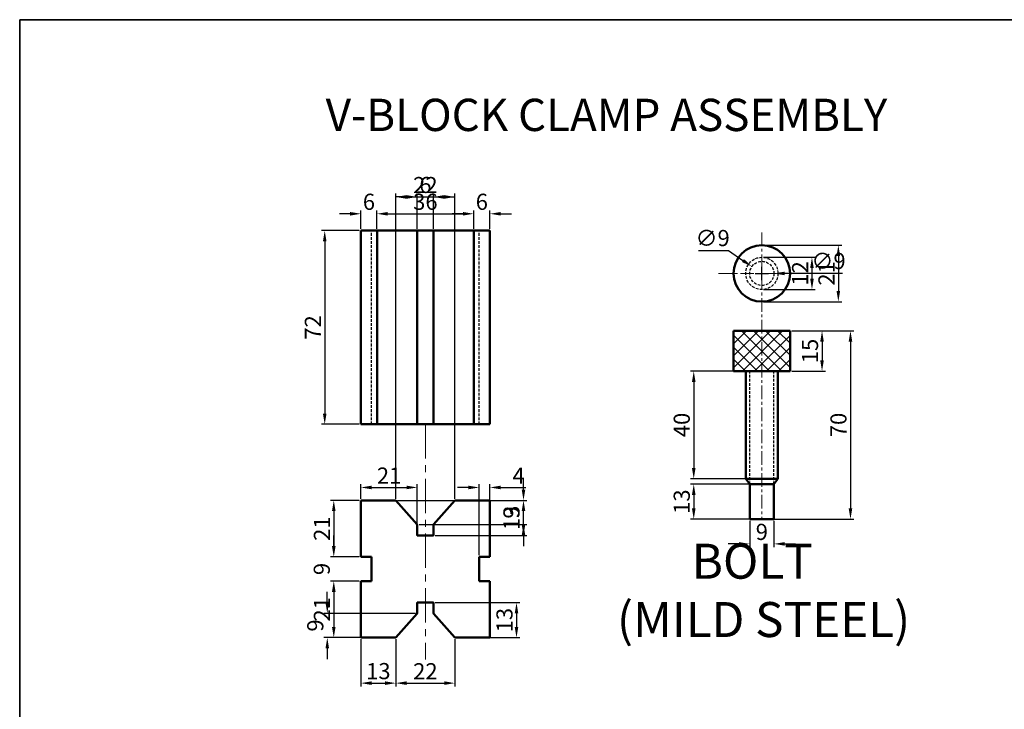
# Model space of a CAD drawing. Units: millimetres. Extents: x 0 to 624, y -214 to 340.
# Tile 2 of 3: x 0 to 366, y 84 to 340. Entities that reach past the tile are written whole.
import ezdxf

# ---------------------------------------------------------------- set-up
doc = ezdxf.new("R2010")
doc.units = ezdxf.units.MM
doc.header["$LTSCALE"] = 0.4
doc.linetypes.add('CENTER', pattern=[50.8, 31.75, -6.35, 6.35, -6.35])
doc.linetypes.add('HIDDEN', pattern=[9.525, 6.35, -3.175])
for name, color, linetype, lineweight in [('M-CNTR', 1, 'CENTER', 18), ('M-DIMS', 2, 'Continuous', 25), ('M-HATC', 8, 'Continuous', 18), ('M-HIDN', 4, 'HIDDEN', 25), ('M-OUTL', 7, 'Continuous', 50), ('M-TEXT', 3, 'Continuous', 25), ('M-TTLB', 7, 'Continuous', 35)]:
    doc.layers.add(name, color=color, linetype=linetype, lineweight=lineweight)
doc.styles.get("Standard").update_dxf_attribs({"font": 'arial.ttf'})
doc.dimstyles.new('ISO-25', dxfattribs={"dimtxt": 6, "dimasz": 4, "dimexe": 1.25, "dimexo": 0.625, "dimtad": 1, "dimtoh": 1, "dimtxsty": 'Standard', "dimcen": 2.5, "dimadec": 0, "dimazin": 0, "dimtfac": 1, "dimtofl": 0, "dimtmove": 0, "dimatfit": 3, "dimfxl": 1, "dimarcsym": 0})

# ---------------------------------------------------------------- blocks, each defined once
blk = doc.blocks.new('*D1')
at = {"layer": 'Defpoints', "color": 0, "transparency": 16777216}
for p in [(126.92, 110.45), (139.92, 110.45), (139.92, 93.53)]:
    blk.add_point(p, dxfattribs=at)
at = {"layer": 'M-DIMS', "color": 0, "lineweight": -2, "transparency": 16777216}
for p, q in [((126.92, 109.83), (126.92, 92.28)), ((139.92, 109.83), (139.92, 92.28)), ((130.92, 93.53), (135.92, 93.53))]:
    blk.add_line(p, q, dxfattribs=at)
at = {"layer": 'M-DIMS', "color": 0, "transparency": 16777216}
for points in [[(130.92, 94.2), (130.92, 92.86), (126.92, 93.53)], [(135.92, 94.2), (135.92, 92.86), (139.92, 93.53)]]:
    blk.add_solid(points, dxfattribs=at)
at = {"layer": 'M-DIMS', "color": 0, "transparency": 16777216, "insert": (133.42, 97.22), "char_height": 6, "attachment_point": 5}
blk.add_mtext('13', dxfattribs=at)
blk = doc.blocks.new('*D2')
at = {"layer": 'Defpoints', "color": 0, "transparency": 16777216}
for p in [(139.92, 110.45), (161.92, 110.45), (161.92, 93.53)]:
    blk.add_point(p, dxfattribs=at)
at = {"layer": 'M-DIMS', "color": 0, "lineweight": -2, "transparency": 16777216}
for p, q in [((139.92, 109.83), (139.92, 92.28)), ((161.92, 109.83), (161.92, 92.28)), ((143.92, 93.53), (157.92, 93.53))]:
    blk.add_line(p, q, dxfattribs=at)
at = {"layer": 'M-DIMS', "color": 0, "transparency": 16777216}
for points in [[(143.92, 94.2), (143.92, 92.86), (139.92, 93.53)], [(157.92, 94.2), (157.92, 92.86), (161.92, 93.53)]]:
    blk.add_solid(points, dxfattribs=at)
at = {"layer": 'M-DIMS', "color": 0, "transparency": 16777216, "insert": (150.92, 97.17), "char_height": 6, "attachment_point": 5}
blk.add_mtext('22', dxfattribs=at)
blk = doc.blocks.new('*D3')
at = {"layer": 'Defpoints', "color": 0, "ltscale": 0.4, "transparency": 16777216}
for p in [(153.92, 123.45), (161.92, 110.45), (184.82, 110.45)]:
    blk.add_point(p, dxfattribs=at)
at = {"layer": 'M-DIMS', "color": 0, "lineweight": -2, "ltscale": 0.4, "transparency": 16777216}
for p, q in [((154.55, 123.45), (186.07, 123.45)), ((184.82, 119.45), (184.82, 114.45)), ((162.55, 110.45), (186.07, 110.45))]:
    blk.add_line(p, q, dxfattribs=at)
at = {"layer": 'M-DIMS', "color": 0, "ltscale": 0.4, "transparency": 16777216}
for points in [[(184.15, 119.45), (185.48, 119.45), (184.82, 123.45)], [(184.15, 114.45), (185.48, 114.45), (184.82, 110.45)]]:
    blk.add_solid(points, dxfattribs=at)
at = {"layer": 'M-DIMS', "color": 0, "ltscale": 0.4, "transparency": 16777216, "insert": (181.13, 116.95), "char_height": 6, "attachment_point": 5, "rotation": 90}
blk.add_mtext('13', dxfattribs=at)
blk = doc.blocks.new('*D4')
at = {"layer": 'Defpoints', "color": 0, "ltscale": 0.4, "transparency": 16777216}
for p in [(174.92, 166.26), (170.92, 140.45), (174.92, 140.45)]:
    blk.add_point(p, dxfattribs=at)
at = {"layer": 'M-DIMS', "color": 0, "lineweight": -2, "ltscale": 0.4, "transparency": 16777216}
for p, q in [((166.92, 166.26), (162.92, 166.26)), ((170.92, 141.08), (170.92, 167.51)), ((174.92, 141.08), (174.92, 167.51)), ((178.92, 166.26), (188.32, 166.26))]:
    blk.add_line(p, q, dxfattribs=at)
at = {"layer": 'M-DIMS', "color": 0, "ltscale": 0.4, "transparency": 16777216}
for points in [[(166.92, 166.92), (166.92, 165.59), (170.92, 166.26)], [(178.92, 166.92), (178.92, 165.59), (174.92, 166.26)]]:
    blk.add_solid(points, dxfattribs=at)
at = {"layer": 'M-DIMS', "color": 0, "ltscale": 0.4, "transparency": 16777216, "insert": (185.62, 169.88), "char_height": 6, "attachment_point": 5}
blk.add_mtext('4', dxfattribs=at)
blk = doc.blocks.new('*D5')
at = {"layer": 'Defpoints', "color": 0, "ltscale": 0.4, "transparency": 16777216}
for p in [(126.92, 161.45), (116.84, 140.45), (126.92, 140.45)]:
    blk.add_point(p, dxfattribs=at)
at = {"layer": 'M-DIMS', "color": 0, "lineweight": -2, "ltscale": 0.4, "transparency": 16777216}
for p, q in [((126.3, 161.45), (115.59, 161.45)), ((116.84, 157.45), (116.84, 144.45)), ((126.3, 140.45), (115.59, 140.45))]:
    blk.add_line(p, q, dxfattribs=at)
at = {"layer": 'M-DIMS', "color": 0, "ltscale": 0.4, "transparency": 16777216}
for points in [[(116.18, 157.45), (117.51, 157.45), (116.84, 161.45)], [(116.18, 144.45), (117.51, 144.45), (116.84, 140.45)]]:
    blk.add_solid(points, dxfattribs=at)
at = {"layer": 'M-DIMS', "color": 0, "ltscale": 0.4, "transparency": 16777216, "insert": (113.21, 150.95), "char_height": 6, "attachment_point": 5, "rotation": 90}
blk.add_mtext('21', dxfattribs=at)
blk = doc.blocks.new('*D6')
at = {"layer": 'Defpoints', "color": 0, "ltscale": 0.4, "transparency": 16777216}
for p in [(126.92, 140.45), (116.84, 131.45), (126.92, 131.45)]:
    blk.add_point(p, dxfattribs=at)
at = {"layer": 'M-DIMS', "color": 0, "lineweight": -2, "ltscale": 0.4, "transparency": 16777216}
for p, q in [((116.84, 144.45), (116.84, 148.45)), ((126.3, 140.45), (115.59, 140.45)), ((126.3, 131.45), (115.59, 131.45)), ((116.84, 127.45), (116.84, 123.45))]:
    blk.add_line(p, q, dxfattribs=at)
at = {"layer": 'M-DIMS', "color": 0, "ltscale": 0.4, "transparency": 16777216}
for points in [[(116.18, 144.45), (117.51, 144.45), (116.84, 140.45)], [(116.18, 127.45), (117.51, 127.45), (116.84, 131.45)]]:
    blk.add_solid(points, dxfattribs=at)
at = {"layer": 'M-DIMS', "color": 0, "ltscale": 0.4, "transparency": 16777216, "insert": (113.16, 135.95), "char_height": 6, "attachment_point": 5, "rotation": 90}
blk.add_mtext('9', dxfattribs=at)
blk = doc.blocks.new('*D7')
at = {"layer": 'Defpoints', "color": 0, "ltscale": 0.4, "transparency": 16777216}
for p in [(126.92, 131.45), (116.84, 110.45), (126.92, 110.45)]:
    blk.add_point(p, dxfattribs=at)
at = {"layer": 'M-DIMS', "color": 0, "lineweight": -2, "ltscale": 0.4, "transparency": 16777216}
for p, q in [((126.3, 131.45), (115.59, 131.45)), ((116.84, 127.45), (116.84, 114.45)), ((126.3, 110.45), (115.59, 110.45))]:
    blk.add_line(p, q, dxfattribs=at)
at = {"layer": 'M-DIMS', "color": 0, "ltscale": 0.4, "transparency": 16777216}
for points in [[(116.18, 127.45), (117.51, 127.45), (116.84, 131.45)], [(116.18, 114.45), (117.51, 114.45), (116.84, 110.45)]]:
    blk.add_solid(points, dxfattribs=at)
at = {"layer": 'M-DIMS', "color": 0, "ltscale": 0.4, "transparency": 16777216, "insert": (113.21, 120.95), "char_height": 6, "attachment_point": 5, "rotation": 90}
blk.add_mtext('21', dxfattribs=at)
blk = doc.blocks.new('*D8')
at = {"layer": 'Defpoints', "color": 0, "ltscale": 0.4, "transparency": 16777216}
for p in [(147.92, 166.26), (126.92, 161.45), (147.92, 148.45)]:
    blk.add_point(p, dxfattribs=at)
at = {"layer": 'M-DIMS', "color": 0, "lineweight": -2, "ltscale": 0.4, "transparency": 16777216}
for p, q in [((126.92, 162.08), (126.92, 167.51)), ((130.92, 166.26), (143.92, 166.26)), ((147.92, 149.08), (147.92, 167.51))]:
    blk.add_line(p, q, dxfattribs=at)
at = {"layer": 'M-DIMS', "color": 0, "ltscale": 0.4, "transparency": 16777216}
for points in [[(130.92, 166.92), (130.92, 165.59), (126.92, 166.26)], [(143.92, 166.92), (143.92, 165.59), (147.92, 166.26)]]:
    blk.add_solid(points, dxfattribs=at)
at = {"layer": 'M-DIMS', "color": 0, "ltscale": 0.4, "transparency": 16777216, "insert": (137.42, 169.89), "char_height": 6, "attachment_point": 5}
blk.add_mtext('21', dxfattribs=at)
blk = doc.blocks.new('*D9')
at = {"layer": 'Defpoints', "color": 0, "ltscale": 0.4, "transparency": 16777216}
for p in [(132.92, 267.98), (126.92, 261.73), (132.92, 261.73)]:
    blk.add_point(p, dxfattribs=at)
at = {"layer": 'M-DIMS', "color": 0, "lineweight": -2, "ltscale": 0.4, "transparency": 16777216}
for p, q in [((122.92, 267.98), (118.92, 267.98)), ((126.92, 262.36), (126.92, 269.23)), ((132.92, 262.36), (132.92, 269.23)), ((136.92, 267.98), (140.92, 267.98))]:
    blk.add_line(p, q, dxfattribs=at)
at = {"layer": 'M-DIMS', "color": 0, "ltscale": 0.4, "transparency": 16777216}
for points in [[(122.92, 268.64), (122.92, 267.31), (126.92, 267.98)], [(136.92, 268.64), (136.92, 267.31), (132.92, 267.98)]]:
    blk.add_solid(points, dxfattribs=at)
at = {"layer": 'M-DIMS', "color": 0, "ltscale": 0.4, "transparency": 16777216, "insert": (129.92, 271.66), "char_height": 6, "attachment_point": 5}
blk.add_mtext('6', dxfattribs=at)
blk = doc.blocks.new('*D10')
at = {"layer": 'Defpoints', "color": 0, "ltscale": 0.4, "transparency": 16777216}
for p in [(168.92, 267.98), (132.92, 261.73), (168.92, 261.73)]:
    blk.add_point(p, dxfattribs=at)
at = {"layer": 'M-DIMS', "color": 0, "lineweight": -2, "ltscale": 0.4, "transparency": 16777216}
for p, q in [((132.92, 262.36), (132.92, 269.23)), ((136.92, 267.98), (164.92, 267.98)), ((168.92, 262.36), (168.92, 269.23))]:
    blk.add_line(p, q, dxfattribs=at)
at = {"layer": 'M-DIMS', "color": 0, "ltscale": 0.4, "transparency": 16777216}
for points in [[(136.92, 268.64), (136.92, 267.31), (132.92, 267.98)], [(164.92, 268.64), (164.92, 267.31), (168.92, 267.98)]]:
    blk.add_solid(points, dxfattribs=at)
at = {"layer": 'M-DIMS', "color": 0, "ltscale": 0.4, "transparency": 16777216, "insert": (150.92, 271.67), "char_height": 6, "attachment_point": 5}
blk.add_mtext('36', dxfattribs=at)
blk = doc.blocks.new('*D11')
at = {"layer": 'Defpoints', "color": 0, "ltscale": 0.4, "transparency": 16777216}
for p in [(174.92, 267.98), (168.92, 261.73), (174.92, 261.73)]:
    blk.add_point(p, dxfattribs=at)
at = {"layer": 'M-DIMS', "color": 0, "lineweight": -2, "ltscale": 0.4, "transparency": 16777216}
for p, q in [((164.92, 267.98), (160.92, 267.98)), ((168.92, 262.36), (168.92, 269.23)), ((174.92, 262.36), (174.92, 269.23)), ((178.92, 267.98), (182.92, 267.98))]:
    blk.add_line(p, q, dxfattribs=at)
at = {"layer": 'M-DIMS', "color": 0, "ltscale": 0.4, "transparency": 16777216}
for points in [[(164.92, 268.64), (164.92, 267.31), (168.92, 267.98)], [(178.92, 268.64), (178.92, 267.31), (174.92, 267.98)]]:
    blk.add_solid(points, dxfattribs=at)
at = {"layer": 'M-DIMS', "color": 0, "ltscale": 0.4, "transparency": 16777216, "insert": (171.92, 271.66), "char_height": 6, "attachment_point": 5}
blk.add_mtext('6', dxfattribs=at)
blk = doc.blocks.new('*D12')
at = {"layer": 'Defpoints', "color": 0, "ltscale": 0.4, "transparency": 16777216}
for p in [(126.92, 261.73), (113.47, 189.73), (126.92, 189.73)]:
    blk.add_point(p, dxfattribs=at)
at = {"layer": 'M-DIMS', "color": 0, "lineweight": -2, "ltscale": 0.4, "transparency": 16777216}
for p, q in [((126.3, 261.73), (112.22, 261.73)), ((113.47, 257.73), (113.47, 193.73)), ((126.3, 189.73), (112.22, 189.73))]:
    blk.add_line(p, q, dxfattribs=at)
at = {"layer": 'M-DIMS', "color": 0, "ltscale": 0.4, "transparency": 16777216}
for points in [[(112.81, 257.73), (114.14, 257.73), (113.47, 261.73)], [(112.81, 193.73), (114.14, 193.73), (113.47, 189.73)]]:
    blk.add_solid(points, dxfattribs=at)
at = {"layer": 'M-DIMS', "color": 0, "ltscale": 0.4, "transparency": 16777216, "insert": (109.84, 225.73), "char_height": 6, "attachment_point": 5, "rotation": 90}
blk.add_mtext('72', dxfattribs=at)
blk = doc.blocks.new('*D24')
at = {"layer": 'Defpoints', "color": 0, "ltscale": 0.4, "transparency": 16777216}
for p in [(286.58, 224.48), (286.58, 209.48), (298.47, 209.48)]:
    blk.add_point(p, dxfattribs=at)
at = {"layer": 'M-DIMS', "color": 0, "lineweight": -2, "ltscale": 0.4, "transparency": 16777216}
for p, q in [((287.2, 224.48), (299.72, 224.48)), ((298.47, 220.48), (298.47, 213.48)), ((287.2, 209.48), (299.72, 209.48))]:
    blk.add_line(p, q, dxfattribs=at)
at = {"layer": 'M-DIMS', "color": 0, "ltscale": 0.4, "transparency": 16777216}
for points in [[(297.81, 220.48), (299.14, 220.48), (298.47, 224.48)], [(297.81, 213.48), (299.14, 213.48), (298.47, 209.48)]]:
    blk.add_solid(points, dxfattribs=at)
at = {"layer": 'M-DIMS', "color": 0, "ltscale": 0.4, "transparency": 16777216, "insert": (294.78, 216.98), "char_height": 6, "attachment_point": 5, "rotation": 90}
blk.add_mtext('15', dxfattribs=at)
blk = doc.blocks.new('*D25')
at = {"layer": 'Defpoints', "color": 0, "ltscale": 0.4, "transparency": 16777216}
for p in [(286.58, 224.48), (276.08, 154.48), (309.06, 154.48)]:
    blk.add_point(p, dxfattribs=at)
at = {"layer": 'M-DIMS', "color": 0, "lineweight": -2, "ltscale": 0.4, "transparency": 16777216}
for p, q in [((287.2, 224.48), (310.31, 224.48)), ((309.06, 220.48), (309.06, 158.48)), ((276.7, 154.48), (310.31, 154.48))]:
    blk.add_line(p, q, dxfattribs=at)
at = {"layer": 'M-DIMS', "color": 0, "ltscale": 0.4, "transparency": 16777216}
for points in [[(308.39, 220.48), (309.73, 220.48), (309.06, 224.48)], [(308.39, 158.48), (309.73, 158.48), (309.06, 154.48)]]:
    blk.add_solid(points, dxfattribs=at)
at = {"layer": 'M-DIMS', "color": 0, "ltscale": 0.4, "transparency": 16777216, "insert": (305.37, 189.48), "char_height": 6, "attachment_point": 5, "rotation": 90}
blk.add_mtext('70', dxfattribs=at)
blk = doc.blocks.new('*D26')
at = {"layer": 'Defpoints', "color": 0, "ltscale": 0.4, "transparency": 16777216}
for p in [(276.08, 256.31), (276.08, 235.31), (304.55, 235.31)]:
    blk.add_point(p, dxfattribs=at)
at = {"layer": 'M-DIMS', "color": 0, "lineweight": -2, "ltscale": 0.4, "transparency": 16777216}
for p, q in [((276.7, 256.31), (305.8, 256.31)), ((304.55, 252.31), (304.55, 239.31)), ((276.7, 235.31), (305.8, 235.31))]:
    blk.add_line(p, q, dxfattribs=at)
at = {"layer": 'M-DIMS', "color": 0, "ltscale": 0.4, "transparency": 16777216}
for points in [[(303.88, 252.31), (305.21, 252.31), (304.55, 256.31)], [(303.88, 239.31), (305.21, 239.31), (304.55, 235.31)]]:
    blk.add_solid(points, dxfattribs=at)
at = {"layer": 'M-DIMS', "color": 0, "ltscale": 0.4, "transparency": 16777216, "insert": (300.91, 245.81), "char_height": 6, "attachment_point": 5, "rotation": 90}
blk.add_mtext('21', dxfattribs=at)
blk = doc.blocks.new('*D27')
at = {"layer": 'Defpoints', "color": 0, "ltscale": 0.4, "transparency": 16777216}
for p in [(276.08, 251.81), (276.08, 239.81), (294.73, 239.81)]:
    blk.add_point(p, dxfattribs=at)
at = {"layer": 'M-DIMS', "color": 0, "lineweight": -2, "ltscale": 0.4, "transparency": 16777216}
for p, q in [((276.7, 251.81), (295.98, 251.81)), ((294.73, 247.81), (294.73, 243.81)), ((276.7, 239.81), (295.98, 239.81))]:
    blk.add_line(p, q, dxfattribs=at)
at = {"layer": 'M-DIMS', "color": 0, "ltscale": 0.4, "transparency": 16777216}
for points in [[(294.07, 247.81), (295.4, 247.81), (294.73, 251.81)], [(294.07, 243.81), (295.4, 243.81), (294.73, 239.81)]]:
    blk.add_solid(points, dxfattribs=at)
at = {"layer": 'M-DIMS', "color": 0, "ltscale": 0.4, "transparency": 16777216, "insert": (291.1, 245.81), "char_height": 6, "attachment_point": 5, "rotation": 90}
blk.add_mtext('12', dxfattribs=at)
blk = doc.blocks.new('*D28')
at = {"layer": 'Defpoints', "color": 0, "ltscale": 0.4, "transparency": 16777216}
for p in [(272.37, 248.35), (279.79, 243.27)]:
    blk.add_point(p, dxfattribs=at)
at = {"layer": 'M-DIMS', "color": 0, "lineweight": -2, "ltscale": 0.4, "transparency": 16777216}
for p, q in [((252.54, 254.32), (263.64, 254.32)), ((263.64, 254.32), (269.06, 250.61)), ((273.58, 245.81), (278.58, 245.81)), ((276.08, 243.31), (276.08, 248.31))]:
    blk.add_line(p, q, dxfattribs=at)
at = {"layer": 'M-DIMS', "color": 0, "ltscale": 0.4, "transparency": 16777216}
blk.add_solid([(269.44, 251.16), (268.69, 250.06), (272.37, 248.35)], dxfattribs=at)
at = {"layer": 'M-DIMS', "color": 0, "ltscale": 0.4, "transparency": 16777216, "insert": (257.78, 258.18), "char_height": 6, "attachment_point": 5}
blk.add_mtext('∅9', dxfattribs=at)
blk = doc.blocks.new('*D30')
at = {"layer": 'Defpoints', "color": 0, "ltscale": 0.4, "transparency": 16777216}
for p in [(139.92, 161.45), (147.92, 152.45), (187.42, 152.45)]:
    blk.add_point(p, dxfattribs=at)
at = {"layer": 'M-DIMS', "color": 0, "lineweight": -2, "ltscale": 0.4, "transparency": 16777216}
for p, q in [((187.42, 165.45), (187.42, 169.45)), ((140.55, 161.45), (188.67, 161.45)), ((148.55, 152.45), (188.67, 152.45)), ((187.42, 148.45), (187.42, 144.45))]:
    blk.add_line(p, q, dxfattribs=at)
at = {"layer": 'M-DIMS', "color": 0, "ltscale": 0.4, "transparency": 16777216}
for points in [[(186.76, 165.45), (188.09, 165.45), (187.42, 161.45)], [(186.76, 148.45), (188.09, 148.45), (187.42, 152.45)]]:
    blk.add_solid(points, dxfattribs=at)
at = {"layer": 'M-DIMS', "color": 0, "ltscale": 0.4, "transparency": 16777216, "insert": (183.73, 156.95), "char_height": 6, "attachment_point": 5, "rotation": 90}
blk.add_mtext('9', dxfattribs=at)
blk = doc.blocks.new('*D31')
at = {"layer": 'Defpoints', "color": 0, "ltscale": 0.4, "transparency": 16777216}
for p in [(161.92, 161.45), (187.42, 161.45), (153.92, 148.45)]:
    blk.add_point(p, dxfattribs=at)
at = {"layer": 'M-DIMS', "color": 0, "lineweight": -2, "ltscale": 0.4, "transparency": 16777216}
for p, q in [((162.55, 161.45), (188.67, 161.45)), ((187.42, 152.45), (187.42, 157.45)), ((154.55, 148.45), (188.67, 148.45))]:
    blk.add_line(p, q, dxfattribs=at)
at = {"layer": 'M-DIMS', "color": 0, "ltscale": 0.4, "transparency": 16777216}
for points in [[(186.76, 157.45), (188.09, 157.45), (187.42, 161.45)], [(186.76, 152.45), (188.09, 152.45), (187.42, 148.45)]]:
    blk.add_solid(points, dxfattribs=at)
at = {"layer": 'M-DIMS', "color": 0, "ltscale": 0.4, "transparency": 16777216, "insert": (183.73, 154.95), "char_height": 6, "attachment_point": 5, "rotation": 90}
blk.add_mtext('13', dxfattribs=at)
blk = doc.blocks.new('*D32')
at = {"layer": 'Defpoints', "color": 0, "ltscale": 0.4, "transparency": 16777216}
for p in [(153.92, 274.23), (147.92, 261.73), (153.92, 261.73)]:
    blk.add_point(p, dxfattribs=at)
at = {"layer": 'M-DIMS', "color": 0, "lineweight": -2, "ltscale": 0.4, "transparency": 16777216}
for p, q in [((147.92, 262.36), (147.92, 275.48)), ((153.92, 262.36), (153.92, 275.48)), ((143.92, 274.23), (139.92, 274.23)), ((157.92, 274.23), (161.92, 274.23))]:
    blk.add_line(p, q, dxfattribs=at)
at = {"layer": 'M-DIMS', "color": 0, "ltscale": 0.4, "transparency": 16777216}
for points in [[(143.92, 274.9), (143.92, 273.56), (147.92, 274.23)], [(157.92, 274.9), (157.92, 273.56), (153.92, 274.23)]]:
    blk.add_solid(points, dxfattribs=at)
at = {"layer": 'M-DIMS', "color": 0, "ltscale": 0.4, "transparency": 16777216, "insert": (150.92, 277.92), "char_height": 6, "attachment_point": 5}
blk.add_mtext('6', dxfattribs=at)
blk = doc.blocks.new('*D33')
at = {"layer": 'Defpoints', "color": 0, "ltscale": 0.4, "transparency": 16777216}
for p in [(161.92, 274.23), (139.92, 161.45), (161.92, 161.45)]:
    blk.add_point(p, dxfattribs=at)
at = {"layer": 'M-DIMS', "color": 0, "lineweight": -2, "ltscale": 0.4, "transparency": 16777216}
for p, q in [((139.92, 162.08), (139.92, 275.48)), ((161.92, 162.08), (161.92, 275.48)), ((143.92, 274.23), (157.92, 274.23))]:
    blk.add_line(p, q, dxfattribs=at)
at = {"layer": 'M-DIMS', "color": 0, "ltscale": 0.4, "transparency": 16777216}
for points in [[(143.92, 274.9), (143.92, 273.56), (139.92, 274.23)], [(157.92, 274.9), (157.92, 273.56), (161.92, 274.23)]]:
    blk.add_solid(points, dxfattribs=at)
at = {"layer": 'M-DIMS', "color": 0, "ltscale": 0.4, "transparency": 16777216, "insert": (150.92, 277.87), "char_height": 6, "attachment_point": 5}
blk.add_mtext('22', dxfattribs=at)
blk = doc.blocks.new('*D34')
at = {"layer": 'Defpoints', "color": 0, "ltscale": 0.4, "transparency": 16777216}
for p in [(147.92, 119.45), (114.42, 110.45), (139.92, 110.45)]:
    blk.add_point(p, dxfattribs=at)
at = {"layer": 'M-DIMS', "color": 0, "lineweight": -2, "ltscale": 0.4, "transparency": 16777216}
for p, q in [((114.42, 123.45), (114.42, 127.45)), ((147.3, 119.45), (113.17, 119.45)), ((139.3, 110.45), (113.17, 110.45)), ((114.42, 106.45), (114.42, 102.45))]:
    blk.add_line(p, q, dxfattribs=at)
at = {"layer": 'M-DIMS', "color": 0, "ltscale": 0.4, "transparency": 16777216}
for points in [[(113.76, 123.45), (115.09, 123.45), (114.42, 119.45)], [(113.76, 106.45), (115.09, 106.45), (114.42, 110.45)]]:
    blk.add_solid(points, dxfattribs=at)
at = {"layer": 'M-DIMS', "color": 0, "ltscale": 0.4, "transparency": 16777216, "insert": (110.73, 114.95), "char_height": 6, "attachment_point": 5, "rotation": 90}
blk.add_mtext('9', dxfattribs=at)
blk = doc.blocks.new('*D35')
at = {"layer": 'Defpoints', "color": 0, "ltscale": 0.4, "transparency": 16777216}
for p in [(282.08, 209.48), (250.76, 169.48), (282.08, 169.48)]:
    blk.add_point(p, dxfattribs=at)
at = {"layer": 'M-DIMS', "color": 0, "lineweight": -2, "ltscale": 0.4, "transparency": 16777216}
for p, q in [((281.45, 209.48), (249.51, 209.48)), ((250.76, 205.48), (250.76, 173.48)), ((281.45, 169.48), (249.51, 169.48))]:
    blk.add_line(p, q, dxfattribs=at)
at = {"layer": 'M-DIMS', "color": 0, "ltscale": 0.4, "transparency": 16777216}
for points in [[(250.09, 205.48), (251.43, 205.48), (250.76, 209.48)], [(250.09, 173.48), (251.43, 173.48), (250.76, 169.48)]]:
    blk.add_solid(points, dxfattribs=at)
at = {"layer": 'M-DIMS', "color": 0, "ltscale": 0.4, "transparency": 16777216, "insert": (247.07, 189.48), "char_height": 6, "attachment_point": 5, "rotation": 90}
blk.add_mtext('40', dxfattribs=at)
blk = doc.blocks.new('*D36')
at = {"layer": 'Defpoints', "color": 0, "ltscale": 0.4, "transparency": 16777216}
for p in [(280.58, 167.48), (250.76, 154.48), (280.58, 154.48)]:
    blk.add_point(p, dxfattribs=at)
at = {"layer": 'M-DIMS', "color": 0, "lineweight": -2, "ltscale": 0.4, "transparency": 16777216}
for p, q in [((279.95, 167.48), (249.51, 167.48)), ((250.76, 163.48), (250.76, 158.48)), ((279.95, 154.48), (249.51, 154.48))]:
    blk.add_line(p, q, dxfattribs=at)
at = {"layer": 'M-DIMS', "color": 0, "ltscale": 0.4, "transparency": 16777216}
for points in [[(250.09, 163.48), (251.43, 163.48), (250.76, 167.48)], [(250.09, 158.48), (251.43, 158.48), (250.76, 154.48)]]:
    blk.add_solid(points, dxfattribs=at)
at = {"layer": 'M-DIMS', "color": 0, "ltscale": 0.4, "transparency": 16777216, "insert": (247.07, 160.98), "char_height": 6, "attachment_point": 5, "rotation": 90}
blk.add_mtext('13', dxfattribs=at)
blk = doc.blocks.new('*D37')
at = {"layer": 'Defpoints', "color": 0, "ltscale": 0.4, "transparency": 16777216}
for p in [(271.58, 154.48), (280.58, 154.48), (280.58, 145.28)]:
    blk.add_point(p, dxfattribs=at)
at = {"layer": 'M-DIMS', "color": 0, "lineweight": -2, "ltscale": 0.4, "transparency": 16777216}
for p, q in [((271.58, 153.86), (271.58, 144.03)), ((280.58, 153.86), (280.58, 144.03)), ((267.58, 145.28), (263.58, 145.28)), ((284.58, 145.28), (288.58, 145.28))]:
    blk.add_line(p, q, dxfattribs=at)
at = {"layer": 'M-DIMS', "color": 0, "ltscale": 0.4, "transparency": 16777216}
for points in [[(267.58, 145.95), (267.58, 144.62), (271.58, 145.28)], [(284.58, 145.95), (284.58, 144.62), (280.58, 145.28)]]:
    blk.add_solid(points, dxfattribs=at)
at = {"layer": 'M-DIMS', "color": 0, "ltscale": 0.4, "transparency": 16777216, "insert": (276.08, 148.97), "char_height": 6, "attachment_point": 5}
blk.add_mtext('9', dxfattribs=at)
blk = doc.blocks.new('*D40')
at = {"layer": 'Defpoints', "color": 0, "ltscale": 0.4, "transparency": 16777216}
for p in [(271.58, 245.82), (280.58, 245.81)]:
    blk.add_point(p, dxfattribs=at)
at = {"layer": 'M-DIMS', "color": 0, "lineweight": -2, "ltscale": 0.4, "transparency": 16777216}
for p, q in [((273.58, 245.81), (278.58, 245.81)), ((276.08, 243.31), (276.08, 248.31)), ((295.04, 245.8), (284.58, 245.81)), ((306.14, 245.8), (295.04, 245.8))]:
    blk.add_line(p, q, dxfattribs=at)
at = {"layer": 'M-DIMS', "color": 0, "ltscale": 0.4, "transparency": 16777216}
blk.add_solid([(284.58, 246.47), (284.58, 245.14), (280.58, 245.81)], dxfattribs=at)
at = {"layer": 'M-DIMS', "color": 0, "ltscale": 0.4, "transparency": 16777216, "insert": (300.9, 249.65), "char_height": 6, "attachment_point": 5}
blk.add_mtext('∅9', dxfattribs=at)

msp = doc.modelspace()

# ---------------------------------------------------------------- hatches: boundary and pattern name
at = {"layer": 'M-HATC', "ltscale": 0.4}
h = msp.add_hatch(dxfattribs=at)
h.set_pattern_fill('ANSI37', color=256)
h.set_pattern_definition([(45, (-222.246, 55.1635), (-2.245064, 2.245064), []), (135, (-222.246, 55.1635), (-2.245064, -2.245064), [])])
h.paths.add_polyline_path([(265.58, 209.482), (286.58, 209.482), (286.58, 224.482), (265.58, 224.482)])

# ---------------------------------------------------------------- linework, layer by layer
at = {"layer": 'M-CNTR', "ltscale": 0.4}
for p, q in [((276.08, 261.013), (276.08, 154.482)), ((259.959, 245.814), (291.416, 245.814))]:
    msp.add_line(p, q, dxfattribs=at)
at = {"layer": 'M-CNTR'}
msp.add_line((150.923, 189.731), (150.923, 102.363), dxfattribs=at)
at = {"layer": 'M-HIDN', "ltscale": 0.4}
for p, q in [((130.923, 189.731), (130.923, 261.731)), ((139.923, 189.731), (139.923, 261.731)), ((161.923, 189.731), (161.923, 261.731)), ((170.923, 189.731), (170.923, 261.731)), ((271.58, 167.482), (271.58, 209.482)), ((280.58, 167.482), (280.58, 209.482))]:
    msp.add_line(p, q, dxfattribs=at)
for radius in [6, 4.5]:
    msp.add_circle((276.08, 245.814), radius, dxfattribs=at)
at = {"layer": 'M-OUTL', "ltscale": 0.4}
for p, q in [((174.923, 261.731), (126.923, 261.731)), ((126.923, 261.731), (126.923, 189.731)), ((132.923, 261.731), (132.923, 189.731)), ((147.923, 189.731), (147.923, 261.731)), ((153.923, 189.731), (153.923, 261.731)), ((168.923, 189.731), (168.923, 261.731)), ((174.923, 189.731), (174.923, 261.731)), ((286.58, 224.482), (265.58, 224.482)), ((265.58, 224.482), (265.58, 209.482)), ((286.58, 209.482), (286.58, 224.482)), ((265.58, 209.482), (286.58, 209.482)), ((270.08, 209.482), (270.08, 169.482)), ((282.08, 169.482), (282.08, 209.482)), ((126.923, 189.731), (150.923, 189.731)), ((150.923, 189.731), (174.923, 189.731)), ((280.58, 169.482), (270.08, 169.482)), ((270.08, 169.482), (271.58, 167.482)), ((282.08, 169.482), (280.58, 169.482)), ((282.08, 169.482), (280.58, 167.482)), ((271.58, 154.482), (271.58, 167.482)), ((280.58, 167.482), (271.58, 167.482)), ((280.58, 154.482), (280.58, 167.482)), ((276.08, 154.482), (271.58, 154.482)), ((276.08, 154.482), (280.58, 154.482)), ((147.923, 148.451), (147.923, 152.451)), ((153.923, 148.451), (153.923, 152.451))]:
    msp.add_line(p, q, dxfattribs=at)
at = {"layer": 'M-OUTL'}
for p, q in [((126.923, 161.451), (126.923, 140.451)), ((139.923, 161.451), (126.923, 161.451)), ((174.923, 161.451), (161.923, 161.451)), ((174.923, 140.451), (174.923, 161.451)), ((126.923, 140.451), (130.923, 140.451)), ((130.923, 140.451), (130.923, 131.451)), ((170.923, 131.451), (170.923, 140.451)), ((170.923, 140.451), (174.923, 140.451)), ((130.923, 131.451), (126.923, 131.451)), ((126.923, 131.451), (126.923, 110.451)), ((174.923, 131.451), (170.923, 131.451)), ((174.923, 110.451), (174.923, 131.451)), ((126.923, 123.451), (126.923, 110.451)), ((126.923, 110.451), (139.923, 110.451)), ((161.923, 110.451), (174.923, 110.451))]:
    msp.add_line(p, q, dxfattribs=at)
for points in [[(139.923, 161.451), (147.923, 152.451), (147.923, 148.451), (150.923, 148.451), (153.923, 148.451), (153.923, 152.451), (161.923, 161.451)], [(139.923, 110.451), (147.923, 119.451), (147.923, 123.451), (150.923, 123.451), (153.923, 123.451), (153.923, 119.451), (161.923, 110.451)]]:
    msp.add_lwpolyline(points, dxfattribs=at)
at = {"layer": 'M-OUTL', "ltscale": 0.4}
msp.add_circle((276.08, 245.814), 10.5, dxfattribs=at)
at = {"layer": 'M-TTLB', "ltscale": 0.4}
msp.add_lwpolyline([(0, 340.107), (623.623, 340.107), (623.623, -214.379), (0, -214.379)], close=True, dxfattribs=at)

# ---------------------------------------------------------------- texts
at = {"layer": 'M-TEXT', "ltscale": 0.4, "attachment_point": 1}
for s, width, insert, char_height in [('V-BLOCK CLAMP ASSEMBLY', 248.23963, (113.826, 310.731), 12), ('           BOLT\\P    (MILD STEEL)', 160.14315, (206.287, 145.342), 13)]:
    msp.add_mtext_dynamic_manual_height_columns(s, width=width, gutter_width=12.5, heights=[0], dxfattribs=dict(at, insert=insert, char_height=char_height))

# ---------------------------------------------------------------- dimensions: what is measured, and where the dimension line sits
at = {"layer": 'M-DIMS', "ltscale": 0.4}
for base, p1, p2, override, picture, middle in [((153.923, 274.231), (147.923, 261.731), (153.923, 261.731), {"dimdec": 0, "dimlfac": 1, "dimrnd": 0, "dimzin": 0, "dimdsep": 46, "dimlunit": 2}, '*D32', (150.923, 277.919)), ((161.923, 274.231), (139.923, 161.451), (161.923, 161.451), {"dimdec": 0, "dimlfac": 1, "dimrnd": 0, "dimzin": 0, "dimdsep": 46, "dimlunit": 2}, '*D33', (150.923, 277.868)), ((132.923, 267.976), (126.923, 261.731), (132.923, 261.731), {"dimclrd": 0, "dimclre": 0, "dimclrt": 0}, '*D9', (129.923, 271.665)), ((168.923, 267.976), (132.923, 261.731), (168.923, 261.731), {"dimclrd": 0, "dimclre": 0, "dimclrt": 0}, '*D10', (150.923, 271.667)), ((174.923, 267.976), (168.923, 261.731), (174.923, 261.731), {"dimclrd": 0, "dimclre": 0, "dimclrt": 0}, '*D11', (171.923, 271.665)), ((147.923, 166.256), (126.923, 161.451), (147.923, 148.451), {"dimclrd": 0, "dimclre": 0, "dimclrt": 0}, '*D8', (137.423, 169.893)), ((174.923, 166.256), (170.923, 140.451), (174.923, 140.451), {"dimclrd": 0, "dimclre": 0, "dimclrt": 0}, '*D4', (185.623, 169.881)), ((280.58, 145.282), (271.58, 154.482), (280.58, 154.482), {"dimdec": 0, "dimlfac": 1, "dimrnd": 0, "dimzin": 0, "dimdsep": 46, "dimlunit": 2}, '*D37', (276.08, 148.97))]:
    dim = msp.add_linear_dim(base=base, p1=p1, p2=p2, dimstyle='ISO-25', override=override, dxfattribs=at)
    dim.commit()
    dim.dimension.update_dxf_attribs({"geometry": picture, "text_midpoint": middle})
for base, p1, p2, override, picture, middle in [((113.474, 189.731), (126.923, 261.731), (126.923, 189.731), {"dimclrd": 0, "dimclre": 0, "dimclrt": 0}, '*D12', (109.837, 225.731)), ((304.545, 235.314), (276.08, 256.314), (276.08, 235.314), {"dimclrd": 0, "dimclre": 0, "dimclrt": 0}, '*D26', (300.908, 245.814)), ((294.735, 239.814), (276.08, 251.814), (276.08, 239.814), {"dimclrd": 0, "dimclre": 0, "dimclrt": 0}, '*D27', (291.098, 245.814)), ((309.059, 154.482), (286.58, 224.482), (276.08, 154.482), {"dimclrd": 0, "dimclre": 0, "dimclrt": 0}, '*D25', (305.37, 189.482)), ((298.472, 209.482), (286.58, 224.482), (286.58, 209.482), {"dimclrd": 0, "dimclre": 0, "dimclrt": 0}, '*D24', (294.784, 216.982)), ((250.76, 169.482), (282.08, 209.482), (282.08, 169.482), {"dimdec": 0, "dimlfac": 1, "dimrnd": 0, "dimzin": 0, "dimdsep": 46, "dimlunit": 2}, '*D35', (247.071, 189.482)), ((187.423, 152.451), (139.923, 161.451), (147.923, 152.451), {"dimdec": 0, "dimlfac": 1, "dimrnd": 0, "dimzin": 0, "dimdsep": 46, "dimlunit": 2}, '*D30', (183.735, 156.951)), ((250.76, 154.482), (280.58, 167.482), (280.58, 154.482), {"dimdec": 0, "dimlfac": 1, "dimrnd": 0, "dimzin": 0, "dimdsep": 46, "dimlunit": 2}, '*D36', (247.069, 160.982)), ((116.845, 140.451), (126.923, 161.451), (126.923, 140.451), {"dimclrd": 0, "dimclre": 0, "dimclrt": 0}, '*D5', (113.207, 150.951)), ((187.423, 161.451), (153.923, 148.451), (161.923, 161.451), {"dimdec": 0, "dimlfac": 1, "dimrnd": 0, "dimzin": 0, "dimdsep": 46, "dimlunit": 2}, '*D31', (183.733, 154.951)), ((116.845, 131.451), (126.923, 140.451), (126.923, 131.451), {"dimclrd": 0, "dimclre": 0, "dimclrt": 0}, '*D6', (113.156, 135.951)), ((116.845, 110.451), (126.923, 131.451), (126.923, 110.451), {"dimclrd": 0, "dimclre": 0, "dimclrt": 0}, '*D7', (113.207, 120.951)), ((114.423, 110.451), (147.923, 119.451), (139.923, 110.451), {"dimdec": 0, "dimlfac": 1, "dimrnd": 0, "dimzin": 0, "dimdsep": 46, "dimlunit": 2}, '*D34', (110.735, 114.951)), ((184.816, 110.451), (153.923, 123.451), (161.923, 110.451), {"dimclrd": 0, "dimclre": 0, "dimclrt": 0}, '*D3', (181.126, 116.951))]:
    dim = msp.add_linear_dim(base=base, p1=p1, p2=p2, angle=90, dimstyle='ISO-25', override=override, dxfattribs=at)
    dim.commit()
    dim.dimension.update_dxf_attribs({"geometry": picture, "text_midpoint": middle})
for p1, p2, override, picture, middle in [((279.794, 243.273), (272.366, 248.355), {"dimclrd": 0, "dimclre": 0, "dimclrt": 0}, '*D28', (257.78, 254.324)), ((271.58, 245.818), (280.58, 245.81), {"dimdec": 0, "dimlfac": 1, "dimrnd": 0, "dimzin": 0, "dimdsep": 46, "dimlunit": 2}, '*D40', (295.042, 245.798))]:
    dim = msp.add_diameter_dim_2p(p1=p1, p2=p2, dimstyle='ISO-25', override=override, dxfattribs=at)
    dim.commit()
    dim.dimension.update_dxf_attribs({"geometry": picture, "text_midpoint": middle, "dimtype": 163})
at = {"layer": 'M-DIMS'}
dim = msp.add_linear_dim(base=(139.923, 93.531), p1=(126.923, 110.451), p2=(139.923, 110.451), dimstyle='ISO-25', override={"dimclrd": 0, "dimclre": 0, "dimclrt": 0}, dxfattribs=at)
dim.commit()
dim.dimension.update_dxf_attribs({"geometry": '*D1', "text_midpoint": (133.423, 93.531), "dimtype": 160})
dim = msp.add_linear_dim(base=(161.923, 93.531), p1=(139.923, 110.451), p2=(161.923, 110.451), dimstyle='ISO-25', override={"dimclrd": 0, "dimclre": 0, "dimclrt": 0}, dxfattribs=at)
dim.commit()
dim.dimension.update_dxf_attribs({"geometry": '*D2', "text_midpoint": (150.923, 97.169)})

doc.saveas('drawing.dxf')
